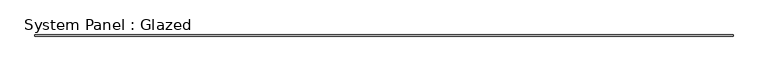
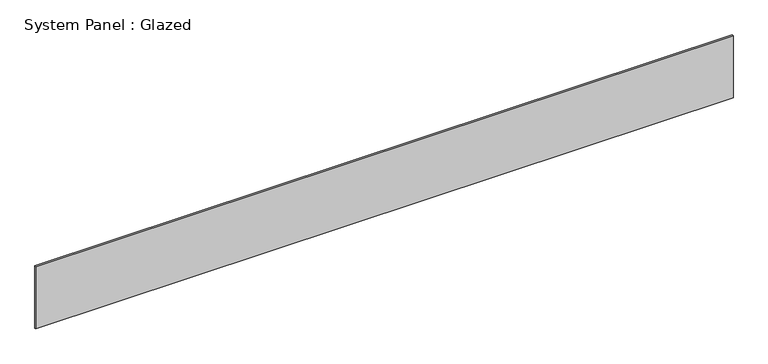
"""IFC4 building model written with IfcOpenShell, lengths in millimetres: plate geometry, System Panel : Glazed."""

from ifc_helpers import new_model, si_unit, origin, origin_with_axes, place, context, project, spatial, polyline, outline, extrude, source, transform, mapped, element, save


def system_panel_glazed_0e082344(model_context):
    return source(origin(), model_context, "Body", "SweptSolid", [
        extrude(outline(polyline([(8064.5, 19.05), (-8064.5, 19.05), (-8064.5, 44.45), (8064.5, 44.45), (8064.5, 19.05)])), origin_with_axes(), (0.0, 0.0, 1.0), 1524.0),
    ])


if __name__ == "__main__":
    model = new_model("IFC4")
    model_context = context("Model", 3, world=origin())
    ifc_project = project(units=[si_unit("LENGTHUNIT", "METRE", prefix="MILLI")], contexts=[model_context])
    site = spatial("IfcSite", under=ifc_project)
    building = spatial("IfcBuilding", under=site)
    placement = place(None, origin())
    system_panel_glazed_shape = system_panel_glazed_0e082344(model_context)
    element("IfcPlate", 1, ObjectType="System Panel : Glazed", at=placement, inside=building, context=model_context, shape_type="MappedRepresentation", body=[
        mapped(system_panel_glazed_shape, transform((0.0, 0.0, 0.0), x_axis=(1.0, 0.0, 0.0), y_axis=(0.0, 1.0, 0.0), z_axis=(0.0, 0.0, 1.0))),
    ])
    save(model, "model.ifc")

# Revit data of these elements
# Type "System Panel : Glazed"
#   Construction Type Id = "GSP4R"
#   Analytic Construction = "1/8 in Pilkington single glazing"
#   Visual Light Transmittance = 0.9
#   Solar Heat Gain Coefficient = 0.86
#   Heat Transfer Coefficient (U) = 1.18115 BTU/(h·ft²·°F)
# Element 1 (IfcPlate, "System Panel : Glazed")
#   Materials on its faces: "Glass"
# Materials
#   "Glass": class "Glass", colour RGB 0 128 192, transparency 0.75, Description = "Soda Lime Glass", Cost = 0
